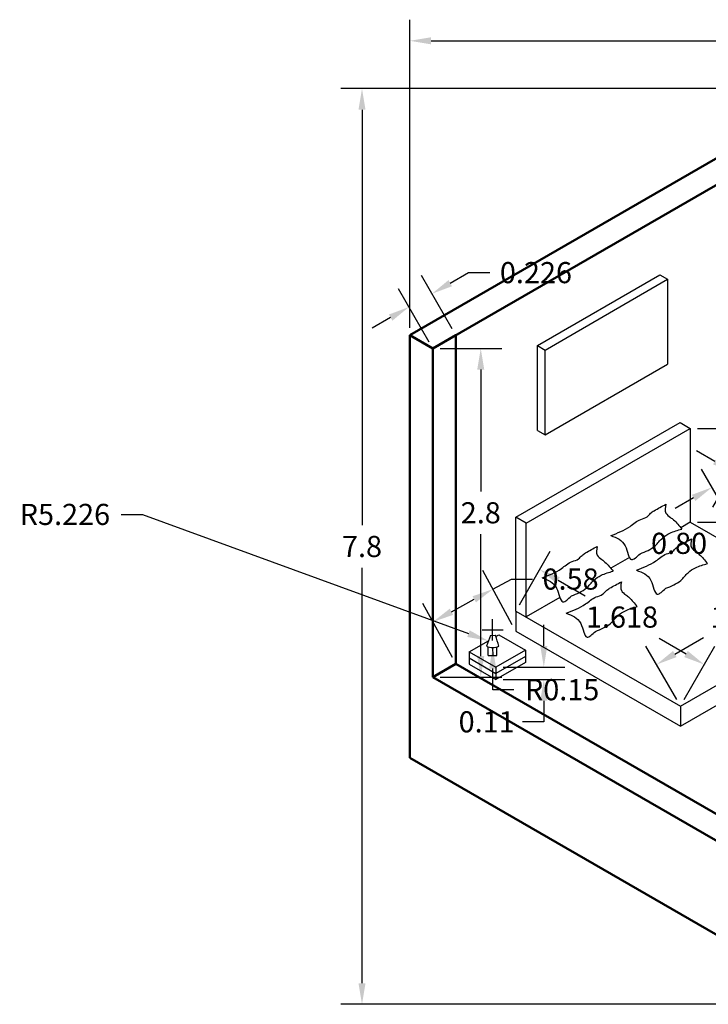
# Model space of a CAD drawing. Units: metres. Extents: x 4633 to 4644.7, y 5356.8 to 5365.2.
# Tile 1 of 3: x 4633 to 4638.8, y 5356.8 to 5365.2. Entities that reach past the tile are written whole.
import ezdxf

# ---------------------------------------------------------------- set-up
doc = ezdxf.new("R2010")
doc.units = ezdxf.units.M
for name, color, linetype, lineweight in [('A-ANNO-DIMS', 2, 'Continuous', 18), ('A-FURN', 8, 'Continuous', 25), ('A-WALL', 7, 'Continuous', 50)]:
    doc.layers.add(name, color=color, linetype=linetype, lineweight=lineweight)
doc.styles.get("Standard").update_dxf_attribs({"font": 'arial.ttf'})
doc.dimstyles.get("Standard").update_dxf_attribs({"dimtxt": 0.18, "dimasz": 0.18, "dimexe": 0.18, "dimexo": 0.0625, "dimgap": 0.09, "dimtad": 0, "dimtih": 1, "dimtoh": 1, "dimdec": 4, "dimzin": 0, "dimdsep": 46, "dimtxsty": 'Standard', "dimcen": 0.09, "dimadec": 0, "dimazin": 0, "dimtfac": 1, "dimtdec": 4, "dimtofl": 0, "dimtmove": 0, "dimatfit": 3, "dimfxl": 1, "dimtolj": 1, "dimtzin": 0, "dimarcsym": 0})

# ---------------------------------------------------------------- blocks, each defined once
blk = doc.blocks.new('PILLOW')
for points, knots in [([(-0.0004, 0.2035), (0.0564, 0.2257), (0.1474, 0.2612), (0.2348, 0.3422), (0.3079, 0.3563), (0.3355, 0.3956), (0.3904, 0.4298), (0.4348, 0.4532), (0.4684, 0.471)], [0, 0, 0, 0, 0.1814257, 0.2905245, 0.349557, 0.391765, 0.4283126, 0.542495, 0.542495, 0.542495, 0.542495]), ([(0.4684, 0.471), (0.4631, 0.4438), (0.454, 0.3971), (0.503, 0.3629), (0.5526, 0.3243), (0.5813, 0.2877), (0.6029, 0.2602)], [0, 0, 0, 0, 0.0748975, 0.1285846, 0.1625, 0.2662858, 0.2662858, 0.2662858, 0.2662858]), ([(0.248, 0.0493), (0.2946, 0.0673), (0.3701, 0.0963), (0.4317, 0.1835), (0.5098, 0.2333), (0.5686, 0.2503), (0.6029, 0.2602)], [0, 0, 0, 0, 0.1456892, 0.2355995, 0.3119916, 0.4186524, 0.4186524, 0.4186524, 0.4186524]), ([(-0.0004, 0.2035), (0.048, 0.1857), (0.1378, 0.1527), (0.1539, -0.0418), (0.2209, 0.0231), (0.248, 0.0493)], [0, 0, 0, 0, 0.1503002, 0.2788499, 0.3660318, 0.3660318, 0.3660318, 0.3660318])]:
    blk.add_open_spline(points, degree=3, knots=knots)
blk = doc.blocks.new('*D2')
at = {"layer": 'A-ANNO-DIMS', "color": 0, "lineweight": -2, "transparency": 16777216}
for p, q in [((4636.2802, 5362.6038), (4636.2802, 5365.2288)), ((4644.0744, 5362.3038), (4644.0744, 5365.2288)), ((4636.4602, 5365.0488), (4639.7847, 5365.0488)), ((4643.8944, 5365.0488), (4640.5699, 5365.0488))]:
    blk.add_line(p, q, dxfattribs=at)
at = {"layer": 'A-ANNO-DIMS', "color": 0, "transparency": 16777216}
for points in [[(4636.4602, 5365.0788), (4636.4602, 5365.0188), (4636.2802, 5365.0488)], [(4643.8944, 5365.0788), (4643.8944, 5365.0188), (4644.0744, 5365.0488)]]:
    blk.add_solid(points, dxfattribs=at)
at = {"layer": 'Defpoints', "color": 0, "transparency": 16777216}
for p in [(4644.0744, 5365.0488), (4636.2802, 5362.5413), (4644.0744, 5362.2413)]:
    blk.add_point(p, dxfattribs=at)
at = {"layer": 'A-ANNO-DIMS', "color": 0, "transparency": 16777216, "insert": (4640.1773, 5365.0488), "char_height": 0.18, "attachment_point": 5}
blk.add_mtext('\\A1;7.794', dxfattribs=at)
blk = doc.blocks.new('*D3')
at = {"layer": 'A-ANNO-DIMS', "color": 0, "lineweight": -2, "transparency": 16777216}
for p, q in [((4639.855, 5364.6413), (4635.6927, 5364.6413)), ((4635.8727, 5364.4613), (4635.8727, 5360.9232)), ((4635.8727, 5357.0213), (4635.8727, 5360.5594)), ((4639.855, 5356.8413), (4635.6927, 5356.8413))]:
    blk.add_line(p, q, dxfattribs=at)
at = {"layer": 'A-ANNO-DIMS', "color": 0, "transparency": 16777216}
for points in [[(4635.8427, 5364.4613), (4635.9027, 5364.4613), (4635.8727, 5364.6413)], [(4635.8427, 5357.0213), (4635.9027, 5357.0213), (4635.8727, 5356.8413)]]:
    blk.add_solid(points, dxfattribs=at)
at = {"layer": 'Defpoints', "color": 0, "transparency": 16777216}
for p in [(4639.9175, 5364.6413), (4635.8727, 5356.8413), (4639.9175, 5356.8413)]:
    blk.add_point(p, dxfattribs=at)
at = {"layer": 'A-ANNO-DIMS', "color": 0, "transparency": 16777216, "insert": (4635.8727, 5360.7413), "char_height": 0.18, "attachment_point": 5}
blk.add_mtext('\\A1;7.8', dxfattribs=at)
blk = doc.blocks.new('*D4')
at = {"layer": 'A-ANNO-DIMS', "color": 0, "lineweight": -2, "transparency": 16777216}
for p, q in [((4636.6238, 5362.9842), (4636.7796, 5363.0742)), ((4636.7796, 5363.0742), (4636.9596, 5363.0742)), ((4636.6404, 5362.5954), (4636.3779, 5363.0501)), ((4636.4447, 5362.4824), (4636.1822, 5362.9371)), ((4636.1163, 5362.6912), (4635.9604, 5362.6012))]:
    blk.add_line(p, q, dxfattribs=at)
at = {"layer": 'A-ANNO-DIMS', "color": 0, "transparency": 16777216}
for points in [[(4636.6088, 5363.0102), (4636.6388, 5362.9582), (4636.4679, 5362.8942)], [(4636.1013, 5362.7172), (4636.1313, 5362.6652), (4636.2722, 5362.7812)]]:
    blk.add_solid(points, dxfattribs=at)
at = {"layer": 'Defpoints', "color": 0, "transparency": 16777216}
for p in [(4636.4679, 5362.8942), (4636.6716, 5362.5413), (4636.4759, 5362.4283)]:
    blk.add_point(p, dxfattribs=at)
at = {"layer": 'A-ANNO-DIMS', "color": 0, "transparency": 16777216, "insert": (4637.3533, 5363.0742), "char_height": 0.18, "attachment_point": 5}
blk.add_mtext('\\A1;0.226', dxfattribs=at)
blk = doc.blocks.new('*D5')
at = {"layer": 'A-ANNO-DIMS', "color": 0, "lineweight": -2, "transparency": 16777216}
for p, q in [((4636.5384, 5362.4283), (4637.0634, 5362.4283)), ((4636.8834, 5362.2483), (4636.8834, 5361.2102)), ((4636.8834, 5359.8083), (4636.8834, 5360.8464)), ((4636.5384, 5359.6283), (4637.0634, 5359.6283))]:
    blk.add_line(p, q, dxfattribs=at)
at = {"layer": 'A-ANNO-DIMS', "color": 0, "transparency": 16777216}
for points in [[(4636.8534, 5362.2483), (4636.9134, 5362.2483), (4636.8834, 5362.4283)], [(4636.8534, 5359.8083), (4636.9134, 5359.8083), (4636.8834, 5359.6283)]]:
    blk.add_solid(points, dxfattribs=at)
at = {"layer": 'Defpoints', "color": 0, "transparency": 16777216}
for p in [(4636.4759, 5362.4283), (4636.4759, 5359.6283), (4636.8834, 5359.6283)]:
    blk.add_point(p, dxfattribs=at)
at = {"layer": 'A-ANNO-DIMS', "color": 0, "transparency": 16777216, "insert": (4636.8834, 5361.0283), "char_height": 0.18, "attachment_point": 5}
blk.add_mtext('\\A1;2.8', dxfattribs=at)
blk = doc.blocks.new('*D17')
at = {"layer": 'A-ANNO-DIMS', "color": 0, "lineweight": -2, "transparency": 16777216}
for p, q in [((4637.213, 5360.2454), (4637.4755, 5360.7001)), ((4637.5414, 5360.4542), (4637.771, 5360.3216)), ((4638.6308, 5359.8252), (4638.4012, 5359.9578)), ((4638.6142, 5359.4364), (4638.8767, 5359.8911))]:
    blk.add_line(p, q, dxfattribs=at)
at = {"layer": 'A-ANNO-DIMS', "color": 0, "transparency": 16777216}
for points in [[(4637.5564, 5360.4802), (4637.5264, 5360.4282), (4637.3855, 5360.5442)], [(4638.6458, 5359.8512), (4638.6158, 5359.7992), (4638.7867, 5359.7352)]]:
    blk.add_solid(points, dxfattribs=at)
at = {"layer": 'Defpoints', "color": 0, "transparency": 16777216}
for p in [(4637.1817, 5360.1913), (4638.7867, 5359.7352), (4638.583, 5359.3823)]:
    blk.add_point(p, dxfattribs=at)
at = {"layer": 'A-ANNO-DIMS', "color": 0, "transparency": 16777216, "insert": (4638.0861, 5360.1397), "char_height": 0.18, "attachment_point": 5}
blk.add_mtext('\\A1;1.618', dxfattribs=at)
blk = doc.blocks.new('*D18')
at = {"layer": 'A-ANNO-DIMS', "color": 0, "lineweight": -2, "transparency": 16777216}
for p, q in [((4639.9499, 5360.2437), (4639.6874, 5360.6983)), ((4639.6215, 5360.4524), (4639.3762, 5360.3108)), ((4638.5351, 5359.8252), (4638.7804, 5359.9668)), ((4638.5517, 5359.4364), (4638.2892, 5359.8911))]:
    blk.add_line(p, q, dxfattribs=at)
at = {"layer": 'A-ANNO-DIMS', "color": 0, "transparency": 16777216}
for points in [[(4639.6065, 5360.4784), (4639.6365, 5360.4265), (4639.7774, 5360.5424)], [(4638.5201, 5359.8512), (4638.5501, 5359.7992), (4638.3792, 5359.7352)]]:
    blk.add_solid(points, dxfattribs=at)
at = {"layer": 'Defpoints', "color": 0, "transparency": 16777216}
for p in [(4639.7774, 5360.5424), (4639.9812, 5360.1895), (4638.583, 5359.3823)]:
    blk.add_point(p, dxfattribs=at)
at = {"layer": 'A-ANNO-DIMS', "color": 0, "transparency": 16777216, "insert": (4639.0783, 5360.1388), "char_height": 0.18, "attachment_point": 5}
blk.add_mtext('\\A1;1.61', dxfattribs=at)
blk = doc.blocks.new('*D20')
at = {"layer": 'A-ANNO-DIMS', "color": 0, "lineweight": -2, "transparency": 16777216}
for p, q in [((4638.7298, 5361.7474), (4639.2548, 5361.7474)), ((4639.0748, 5361.5674), (4639.0748, 5361.1281)), ((4638.7298, 5360.9481), (4639.2548, 5360.9481)), ((4639.0748, 5360.9481), (4639.0748, 5360.7681)), ((4639.0748, 5360.7681), (4638.8948, 5360.7681))]:
    blk.add_line(p, q, dxfattribs=at)
at = {"layer": 'A-ANNO-DIMS', "color": 0, "transparency": 16777216}
for points in [[(4639.0448, 5361.5674), (4639.1048, 5361.5674), (4639.0748, 5361.7474)], [(4639.0448, 5361.1281), (4639.1048, 5361.1281), (4639.0748, 5360.9481)]]:
    blk.add_solid(points, dxfattribs=at)
at = {"layer": 'Defpoints', "color": 0, "transparency": 16777216}
for p in [(4638.6673, 5361.7474), (4638.6673, 5360.9481), (4639.0748, 5360.9481)]:
    blk.add_point(p, dxfattribs=at)
at = {"layer": 'A-ANNO-DIMS', "color": 0, "transparency": 16777216, "insert": (4638.5714, 5360.7681), "char_height": 0.18, "attachment_point": 5}
blk.add_mtext('\\A1;0.80', dxfattribs=at)
blk = doc.blocks.new('*D21')
at = {"layer": 'A-ANNO-DIMS', "color": 0, "lineweight": -2, "transparency": 16777216}
for p, q in [((4637.1518, 5360.0748), (4636.9001, 5360.5355)), ((4636.9864, 5360.3776), (4637.1444, 5360.4638)), ((4637.1444, 5360.4638), (4637.3244, 5360.4638)), ((4636.6342, 5360.1852), (4636.8284, 5360.2913)), ((4636.6417, 5359.7961), (4636.39, 5360.2569))]:
    blk.add_line(p, q, dxfattribs=at)
at = {"layer": 'A-ANNO-DIMS', "color": 0, "transparency": 16777216}
for points in [[(4636.8141, 5360.3176), (4636.8428, 5360.2649), (4636.9864, 5360.3776)], [(4636.6199, 5360.2115), (4636.6486, 5360.1589), (4636.4763, 5360.0989)]]:
    blk.add_solid(points, dxfattribs=at)
at = {"layer": 'Defpoints', "color": 0, "transparency": 16777216}
for p in [(4636.9864, 5360.3776), (4637.1817, 5360.0199), (4636.6716, 5359.7413)]:
    blk.add_point(p, dxfattribs=at)
at = {"layer": 'A-ANNO-DIMS', "color": 0, "transparency": 16777216, "insert": (4637.6483, 5360.4638), "char_height": 0.18, "attachment_point": 5}
blk.add_mtext('\\A1;0.58', dxfattribs=at)
blk = doc.blocks.new('*D22')
at = {"layer": 'A-ANNO-DIMS', "color": 0, "lineweight": -2, "transparency": 16777216}
for p, q in [((4638.8758, 5361.4662), (4638.7199, 5361.5562)), ((4638.8591, 5361.0775), (4639.1216, 5361.5321)), ((4639.0863, 5360.9463), (4639.3488, 5361.401)), ((4639.4147, 5361.1551), (4639.5706, 5361.0651)), ((4639.5706, 5361.0651), (4639.7506, 5361.0651))]:
    blk.add_line(p, q, dxfattribs=at)
at = {"layer": 'A-ANNO-DIMS', "color": 0, "transparency": 16777216}
for points in [[(4638.8908, 5361.4922), (4638.8608, 5361.4403), (4639.0316, 5361.3762)], [(4639.4297, 5361.1811), (4639.3997, 5361.1291), (4639.2588, 5361.2451)]]:
    blk.add_solid(points, dxfattribs=at)
at = {"layer": 'Defpoints', "color": 0, "transparency": 16777216}
for p in [(4639.2588, 5361.2451), (4638.8279, 5361.0233), (4639.0551, 5360.8922)]:
    blk.add_point(p, dxfattribs=at)
at = {"layer": 'A-ANNO-DIMS', "color": 0, "transparency": 16777216, "insert": (4640.0743, 5361.0651), "char_height": 0.18, "attachment_point": 5}
blk.add_mtext('\\A1;0.26', dxfattribs=at)
blk = doc.blocks.new('*D23')
at = {"layer": 'A-ANNO-DIMS', "color": 0, "lineweight": -2, "transparency": 16777216}
for p, q in [((4639.2746, 5361.0911), (4639.0121, 5361.5457)), ((4639.258, 5361.4799), (4639.4139, 5361.5699)), ((4639.4139, 5361.5699), (4639.5939, 5361.5699)), ((4639.0238, 5360.9463), (4638.7613, 5361.401)), ((4638.6954, 5361.1551), (4638.5395, 5361.0651))]:
    blk.add_line(p, q, dxfattribs=at)
at = {"layer": 'A-ANNO-DIMS', "color": 0, "transparency": 16777216}
for points in [[(4639.243, 5361.5058), (4639.273, 5361.4539), (4639.1021, 5361.3899)], [(4638.6804, 5361.1811), (4638.7104, 5361.1291), (4638.8513, 5361.2451)]]:
    blk.add_solid(points, dxfattribs=at)
at = {"layer": 'Defpoints', "color": 0, "transparency": 16777216}
for p in [(4639.1021, 5361.3899), (4639.3058, 5361.037), (4639.0551, 5360.8922)]:
    blk.add_point(p, dxfattribs=at)
at = {"layer": 'A-ANNO-DIMS', "color": 0, "transparency": 16777216, "insert": (4639.9178, 5361.5699), "char_height": 0.18, "attachment_point": 5}
blk.add_mtext('\\A1;0.29', dxfattribs=at)
blk = doc.blocks.new('*D24')
at = {"layer": 'A-ANNO-DIMS', "color": 0, "lineweight": -2, "transparency": 16777216}
for p, q in [((4637.4201, 5359.893), (4637.4201, 5360.073)), ((4637.0751, 5359.713), (4637.6001, 5359.713)), ((4637.0751, 5359.6076), (4637.6001, 5359.6076)), ((4637.4201, 5359.4276), (4637.4201, 5359.2476)), ((4637.4201, 5359.2476), (4637.2401, 5359.2476))]:
    blk.add_line(p, q, dxfattribs=at)
at = {"layer": 'A-ANNO-DIMS', "color": 0, "transparency": 16777216}
for points in [[(4637.3901, 5359.893), (4637.4501, 5359.893), (4637.4201, 5359.713)], [(4637.3901, 5359.4276), (4637.4501, 5359.4276), (4637.4201, 5359.6076)]]:
    blk.add_solid(points, dxfattribs=at)
at = {"layer": 'Defpoints', "color": 0, "transparency": 16777216}
for p in [(4637.0126, 5359.713), (4637.0126, 5359.6076), (4637.4201, 5359.6076)]:
    blk.add_point(p, dxfattribs=at)
at = {"layer": 'A-ANNO-DIMS', "color": 0, "transparency": 16777216, "insert": (4636.9337, 5359.2476), "char_height": 0.18, "attachment_point": 5}
blk.add_mtext('\\A1;0.11', dxfattribs=at)
blk = doc.blocks.new('*D30')
at = {"layer": 'A-ANNO-DIMS', "color": 0, "lineweight": -2, "transparency": 16777216}
for p, q in [((4633.8236, 5361.0144), (4634.0036, 5361.0144)), ((4634.0036, 5361.0144), (4636.779, 5359.9989)), ((4641.8554, 5358.0514), (4641.8554, 5358.2314)), ((4641.7654, 5358.1414), (4641.9454, 5358.1414))]:
    blk.add_line(p, q, dxfattribs=at)
at = {"layer": 'A-ANNO-DIMS', "color": 0, "transparency": 16777216}
blk.add_solid([(4636.7893, 5360.027), (4636.7686, 5359.9707), (4636.948, 5359.937)], dxfattribs=at)
at = {"layer": 'Defpoints', "color": 0, "transparency": 16777216}
for p in [(4636.948, 5359.937), (4641.8554, 5358.1414)]:
    blk.add_point(p, dxfattribs=at)
at = {"layer": 'A-ANNO-DIMS', "color": 0, "transparency": 16777216, "insert": (4633.3438, 5361.0144), "char_height": 0.18, "attachment_point": 5}
blk.add_mtext('\\A1;R5.226', dxfattribs=at)
blk = doc.blocks.new('*D31')
at = {"layer": 'A-ANNO-DIMS', "color": 0, "lineweight": -2, "transparency": 16777216}
for p, q in [((4636.9848, 5359.9413), (4636.9848, 5360.1213)), ((4636.8948, 5360.0313), (4637.0748, 5360.0313)), ((4636.9856, 5359.5213), (4636.9853, 5359.7013)), ((4637.1656, 5359.5213), (4636.9856, 5359.5213))]:
    blk.add_line(p, q, dxfattribs=at)
at = {"layer": 'A-ANNO-DIMS', "color": 0, "transparency": 16777216}
blk.add_solid([(4637.0153, 5359.7013), (4636.9553, 5359.7012), (4636.985, 5359.8813)], dxfattribs=at)
at = {"layer": 'Defpoints', "color": 0, "transparency": 16777216}
for p in [(4636.9848, 5360.0313), (4636.985, 5359.8813)]:
    blk.add_point(p, dxfattribs=at)
at = {"layer": 'A-ANNO-DIMS', "color": 0, "transparency": 16777216, "insert": (4637.5762, 5359.5213), "char_height": 0.18, "attachment_point": 5}
blk.add_mtext('\\A1;R0.15', dxfattribs=at)

msp = doc.modelspace()

# ---------------------------------------------------------------- linework, layer by layer
at = {"layer": 'A-FURN'}
for p, q in [((4637.3655, 5362.4525), (4638.409, 5363.055)), ((4638.409, 5363.055), (4638.4744, 5363.0172)), ((4637.4309, 5362.4147), (4638.4744, 5363.0172)), ((4638.4744, 5363.0172), (4638.4744, 5362.2938)), ((4637.3655, 5361.7291), (4637.3655, 5362.4525)), ((4637.3655, 5362.4525), (4637.4309, 5362.4147)), ((4637.4309, 5361.6913), (4637.4309, 5362.4147)), ((4637.4309, 5361.6913), (4638.4744, 5362.2938)), ((4637.1817, 5360.9907), (4638.5799, 5361.7979)), ((4638.5799, 5361.7979), (4638.6673, 5361.7474)), ((4637.2692, 5360.9402), (4638.6673, 5361.7474)), ((4637.3655, 5361.7291), (4637.4309, 5361.6913)), ((4638.6673, 5361.7474), (4638.6673, 5360.9481)), ((4637.1817, 5360.1913), (4637.1817, 5360.9907)), ((4637.2692, 5360.9402), (4637.1817, 5360.9907)), ((4637.2692, 5360.1408), (4637.2692, 5360.9402)), ((4638.6673, 5360.9481), (4638.5856, 5360.9009)), ((4638.6673, 5360.9481), (4639.9812, 5360.1895)), ((4638.1484, 5360.6485), (4637.9893, 5360.5566)), ((4637.557, 5360.307), (4637.2692, 5360.1408)), ((4637.1817, 5360.1913), (4638.583, 5359.3823)), ((4637.1817, 5360.1913), (4637.1817, 5360.0199)), ((4638.583, 5359.3823), (4639.9812, 5360.1895)), ((4636.9652, 5359.9834), (4637.0094, 5359.9847)), ((4637.0125, 5359.9752), (4637.0362, 5359.9889)), ((4637.0362, 5359.9889), (4637.2634, 5359.8577)), ((4637.1817, 5360.0199), (4638.583, 5359.2109)), ((4638.583, 5359.2109), (4639.9812, 5360.0182)), ((4636.7854, 5359.8441), (4636.9484, 5359.9382)), ((4636.9469, 5359.8115), (4636.9469, 5359.8861)), ((4636.9848, 5359.8813), (4636.9855, 5359.8119)), ((4637.0205, 5359.8123), (4637.0205, 5359.8856)), ((4636.7854, 5359.8441), (4637.0126, 5359.713)), ((4636.7854, 5359.8441), (4636.7854, 5359.7914)), ((4636.7854, 5359.7914), (4637.0126, 5359.6603)), ((4636.7854, 5359.7914), (4637.0126, 5359.6603)), ((4636.7854, 5359.7914), (4636.7854, 5359.7388)), ((4636.9469, 5359.8115), (4637.0205, 5359.8123)), ((4637.2634, 5359.8577), (4637.0126, 5359.713)), ((4637.2634, 5359.8051), (4637.0126, 5359.6603)), ((4637.2634, 5359.8051), (4637.0126, 5359.6603)), ((4637.2634, 5359.8577), (4637.2634, 5359.8051)), ((4637.2634, 5359.8051), (4637.2634, 5359.7524)), ((4636.7854, 5359.7388), (4637.0126, 5359.6076)), ((4637.2634, 5359.7524), (4637.0126, 5359.6076)), ((4637.0126, 5359.713), (4637.0126, 5359.6603)), ((4637.0126, 5359.6603), (4637.0126, 5359.6076)), ((4638.583, 5359.3823), (4638.583, 5359.2109))]:
    msp.add_line(p, q, dxfattribs=at)
for centre, radius, start, end in [((4641.8554, 5358.1414), 5.2256, 159.35961, 160.43799), ((4634.9418, 5359.2995), 2.1782, 15.75868, 18.33582), ((4636.9848, 5360.0313), 0.1501, 249.18314, 290.81686)]:
    msp.add_arc(centre, radius, start, end, dxfattribs=at)
at = {"layer": 'A-WALL'}
for p, q in [((4636.2802, 5362.5413), (4639.9175, 5364.6413)), ((4636.4759, 5362.4283), (4639.9175, 5364.4153)), ((4636.2802, 5358.9413), (4636.2802, 5362.5413)), ((4636.2802, 5362.5413), (4636.4759, 5362.4283)), ((4636.4759, 5362.4283), (4636.6716, 5362.5413)), ((4636.6716, 5359.7413), (4636.6716, 5362.5413)), ((4636.4759, 5359.6283), (4636.4759, 5362.4283)), ((4636.4759, 5359.6283), (4636.6716, 5359.7413)), ((4636.6716, 5359.7413), (4639.9175, 5357.8673)), ((4639.9175, 5357.6413), (4636.4759, 5359.6283)), ((4636.2802, 5358.9413), (4639.9175, 5356.8413))]:
    msp.add_line(p, q, dxfattribs=at)

# ---------------------------------------------------------------- block references
at = {"layer": 'A-FURN'}
for p in [(4637.991, 5360.63), (4638.2097, 5360.3355), (4637.4068, 5360.2708), (4637.612, 5359.969)]:
    msp.add_blockref('PILLOW', p, dxfattribs=at)

# ---------------------------------------------------------------- dimensions: what is measured, and where the dimension line sits
at = {"layer": 'A-ANNO-DIMS'}
dim = msp.add_linear_dim(base=(4644.0744, 5365.0488), p1=(4636.2802, 5362.5413), p2=(4644.0744, 5362.2413), dimstyle='Standard', override={"dimdec": 3, "dimlfac": 1, "dimrnd": 0, "dimzin": 0, "dimdsep": 46, "dimlunit": 2}, dxfattribs=at)
dim.commit()
dim.dimension.update_dxf_attribs({"geometry": '*D2', "text_midpoint": (4640.1773, 5365.0488)})
for base, p1, p2, angle, override, picture, middle in [((4635.8727, 5356.8413), (4639.9175, 5364.6413), (4639.9175, 5356.8413), 90, {"dimdec": 1, "dimlfac": 1, "dimrnd": 0, "dimzin": 0, "dimdsep": 46, "dimlunit": 2}, '*D3', (4635.8727, 5360.7413)), ((4636.4679, 5362.8942), (4636.4759, 5362.4283), (4636.6716, 5362.5413), 30, {"dimdec": 3, "dimlfac": 1, "dimrnd": 0, "dimzin": 0, "dimdsep": 46, "dimlunit": 2}, '*D4', (4637.3533, 5363.0742)), ((4636.8834, 5359.6283), (4636.4759, 5362.4283), (4636.4759, 5359.6283), 270, {"dimdec": 1, "dimlfac": 1, "dimrnd": 0, "dimzin": 0, "dimdsep": 46, "dimlunit": 2}, '*D5', (4636.8834, 5361.0283)), ((4639.0748, 5360.9481), (4638.6673, 5361.7474), (4638.6673, 5360.9481), 270, {"dimdec": 2, "dimlfac": 1, "dimrnd": 0, "dimzin": 0, "dimdsep": 46, "dimlunit": 2}, '*D20', (4638.5714, 5360.7681)), ((4639.1021, 5361.3899), (4639.0551, 5360.8922), (4639.3058, 5361.037), 30, {"dimdec": 2, "dimlfac": 1, "dimrnd": 0, "dimzin": 0, "dimdsep": 46, "dimlunit": 2}, '*D23', (4639.9178, 5361.5699)), ((4639.2588, 5361.2451), (4638.8279, 5361.0233), (4639.0551, 5360.8922), 330, {"dimdec": 2, "dimlfac": 1, "dimrnd": 0, "dimzin": 0, "dimdsep": 46, "dimlunit": 2}, '*D22', (4640.0743, 5361.0651)), ((4638.7867, 5359.7352), (4637.1817, 5360.1913), (4638.583, 5359.3823), 330, {"dimdec": 3, "dimlfac": 1, "dimrnd": 0, "dimzin": 0, "dimdsep": 46, "dimlunit": 2}, '*D17', (4638.0861, 5360.1397)), ((4639.7774, 5360.5424), (4638.583, 5359.3823), (4639.9812, 5360.1895), 30, {"dimdec": 2, "dimlfac": 1, "dimrnd": 0, "dimzin": 0, "dimdsep": 46, "dimlunit": 2}, '*D18', (4639.0783, 5360.1388)), ((4636.9864, 5360.3776), (4636.6716, 5359.7413), (4637.1817, 5360.0199), 28.64504, {"dimdec": 2, "dimlfac": 1, "dimrnd": 0, "dimzin": 0, "dimdsep": 46, "dimlunit": 2}, '*D21', (4637.6483, 5360.4638)), ((4637.4201, 5359.6076), (4637.0126, 5359.713), (4637.0126, 5359.6076), 270, {"dimdec": 2, "dimlfac": 1, "dimrnd": 0, "dimzin": 0, "dimdsep": 46, "dimlunit": 2}, '*D24', (4636.9337, 5359.2476))]:
    dim = msp.add_linear_dim(base=base, p1=p1, p2=p2, angle=angle, dimstyle='Standard', override=override, dxfattribs=at)
    dim.commit()
    dim.dimension.update_dxf_attribs({"geometry": picture, "text_midpoint": middle})
dim = msp.add_radius_dim(center=(4641.8554, 5358.1414), mpoint=(4636.948, 5359.937), dimstyle='Standard', override={"dimdec": 3, "dimlfac": 1, "dimrnd": 0, "dimzin": 0, "dimdsep": 46, "dimlunit": 2}, dxfattribs=at)
dim.commit()
dim.dimension.update_dxf_attribs({"geometry": '*D30', "text_midpoint": (4633.3438, 5361.0144), "dimtype": 164})
dim = msp.add_radius_dim(center=(4636.9848, 5360.0313), mpoint=(4636.985, 5359.8813), dimstyle='Standard', override={"dimdec": 2, "dimlfac": 1, "dimrnd": 0, "dimzin": 0, "dimdsep": 46, "dimlunit": 2}, dxfattribs=at)
dim.commit()
dim.dimension.update_dxf_attribs({"geometry": '*D31', "text_midpoint": (4637.5762, 5359.5213)})

doc.saveas('drawing.dxf')
